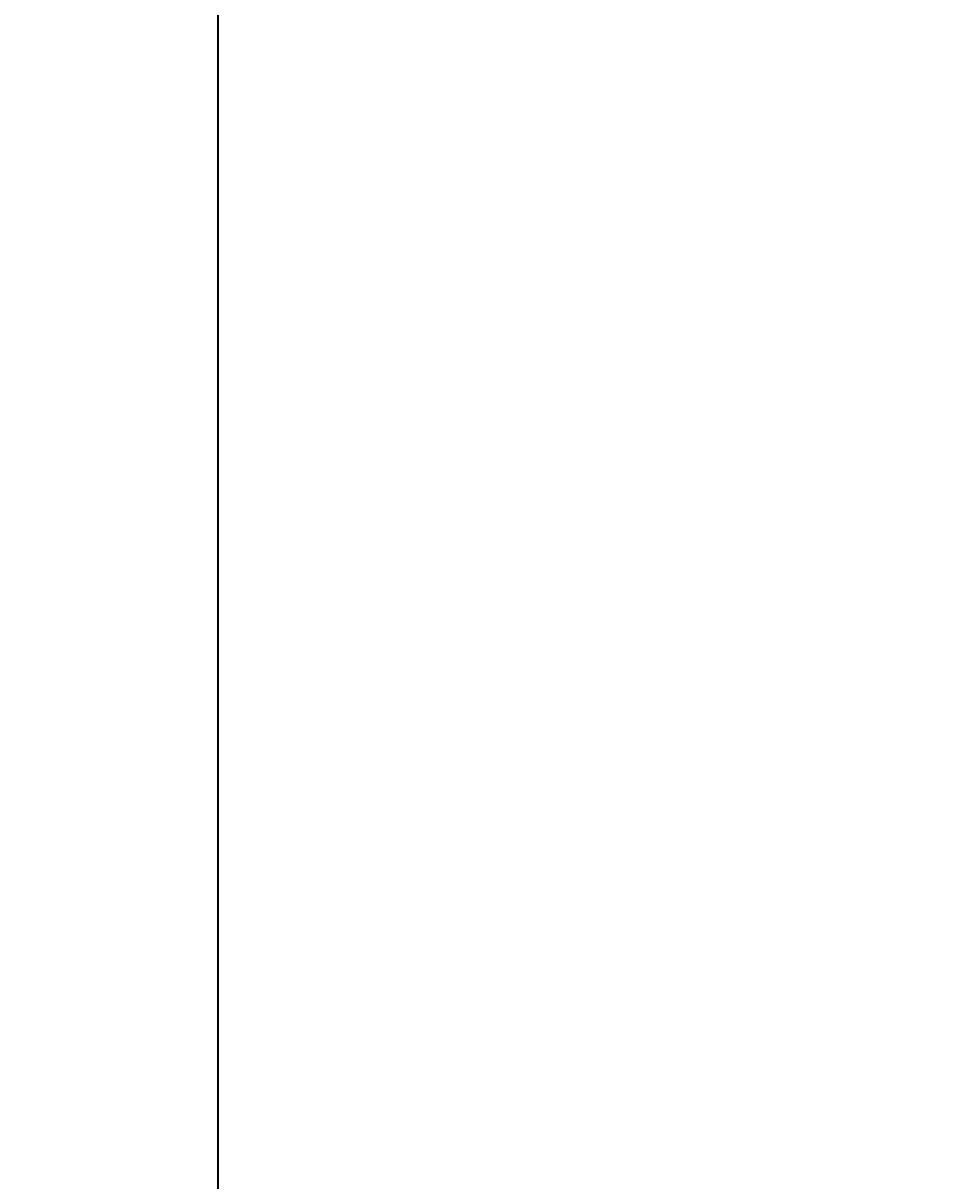
# Model space of a CAD drawing. Units: inches. Extents: x -61 to 1599, y -1316 to 257.
# Tile 98 of 204: x 114 to 142, y -166 to -131. Entities that reach past the tile are written whole.
import ezdxf

# ---------------------------------------------------------------- set-up
doc = ezdxf.new("R2010")
doc.units = ezdxf.units.IN
doc.header["$MEASUREMENT"] = 0
doc.layers.add('A-ANNO-DIMS', color=2, linetype='Continuous', lineweight=18)
doc.layers.add('WALLS', color=4, linetype='Continuous', lineweight=35)
doc.styles.get("Standard").update_dxf_attribs({"font": 'arial.ttf'})
doc.dimstyles.get("Standard").update_dxf_attribs({"dimtxt": 0.18, "dimasz": 0.18, "dimexe": 0.18, "dimexo": 0.0625, "dimgap": 0.09, "dimtad": 0, "dimtih": 1, "dimtoh": 1, "dimdec": 0, "dimzin": 0, "dimdsep": 46, "dimlunit": 3, "dimtxsty": 'Standard', "dimcen": 0.09, "dimadec": 0, "dimazin": 0, "dimtfac": 1, "dimtdec": 0, "dimtofl": 0, "dimtmove": 0, "dimatfit": 3, "dimfxl": 1, "dimtolj": 1, "dimtzin": 0, "dimarcsym": 0})

# ---------------------------------------------------------------- blocks, each defined once
blk = doc.blocks.new('*D687')
at = {"layer": 'A-ANNO-DIMS', "color": 0, "lineweight": -2, "transparency": 16777216}
for p, q in [((289.418, 181.677), (-61.077, 181.677)), ((-60.897, 181.497), (-60.897, -528.952)), ((-60.897, -1239.765), (-60.897, -529.316)), ((319.64, -1239.945), (-61.077, -1239.945))]:
    blk.add_line(p, q, dxfattribs=at)
at = {"layer": 'A-ANNO-DIMS', "color": 0, "transparency": 16777216}
for points in [[(-60.927, 181.497), (-60.867, 181.497), (-60.897, 181.677)], [(-60.927, -1239.765), (-60.867, -1239.765), (-60.897, -1239.945)]]:
    blk.add_solid(points, dxfattribs=at)
at = {"layer": 'DEFPOINTS', "color": 0, "transparency": 16777216}
for p in [(289.481, 181.677), (-60.897, -1239.945), (319.703, -1239.945)]:
    blk.add_point(p, dxfattribs=at)
at = {"layer": 'A-ANNO-DIMS', "color": 0, "transparency": 16777216, "insert": (-60.897, -529.134), "char_height": 0.18, "attachment_point": 5}
blk.add_mtext('\\A1;1421.6', dxfattribs=at)
blk = doc.blocks.new('*D700')
at = {"layer": 'A-ANNO-DIMS', "color": 0, "lineweight": -2, "transparency": 16777216}
for p, q in [((14.703, -616.882), (14.703, 257.457)), ((14.883, 257.277), (96.772, 257.277)), ((179.572, 257.277), (97.683, 257.277)), ((179.752, -616.882), (179.752, 257.457))]:
    blk.add_line(p, q, dxfattribs=at)
at = {"layer": 'A-ANNO-DIMS', "color": 0, "transparency": 16777216}
for points in [[(14.883, 257.307), (14.883, 257.247), (14.703, 257.277)], [(179.572, 257.307), (179.572, 257.247), (179.752, 257.277)]]:
    blk.add_solid(points, dxfattribs=at)
at = {"layer": 'DEFPOINTS', "color": 0, "transparency": 16777216}
for p in [(179.752, 257.277), (14.703, -616.945), (179.752, -616.945)]:
    blk.add_point(p, dxfattribs=at)
at = {"layer": 'A-ANNO-DIMS', "color": 0, "transparency": 16777216, "insert": (97.227, 257.277), "char_height": 0.18, "attachment_point": 5}
blk.add_mtext('\\A1;165.05', dxfattribs=at)

msp = doc.modelspace()

# ---------------------------------------------------------------- linework, layer by layer
at = {"layer": 'WALLS'}
msp.add_line((119.7028, -169.3229), (119.7028, -13.3229), dxfattribs=at)

# ---------------------------------------------------------------- dimensions: what is measured, and where the dimension line sits
at = {"layer": 'A-ANNO-DIMS'}
dim = msp.add_linear_dim(base=(179.7521, 257.2771), p1=(14.7028, -616.9446), p2=(179.7521, -616.9446), dimstyle='Standard', override={"dimdec": 2, "dimlfac": 1, "dimrnd": 0, "dimzin": 0, "dimdsep": 46, "dimlunit": 2}, dxfattribs=at)
dim.commit()
dim.dimension.update_dxf_attribs({"geometry": '*D700', "text_midpoint": (97.2274, 257.2771)})
dim = msp.add_linear_dim(base=(-60.8972, -1239.9446), p1=(289.4807, 181.6771), p2=(319.7028, -1239.9446), angle=90, dimstyle='Standard', override={"dimdec": 1, "dimlfac": 1, "dimrnd": 0, "dimzin": 0, "dimdsep": 46, "dimlunit": 2}, dxfattribs=at)
dim.commit()
dim.dimension.update_dxf_attribs({"geometry": '*D687', "text_midpoint": (-60.8972, -529.1337)})

doc.saveas('drawing.dxf')
